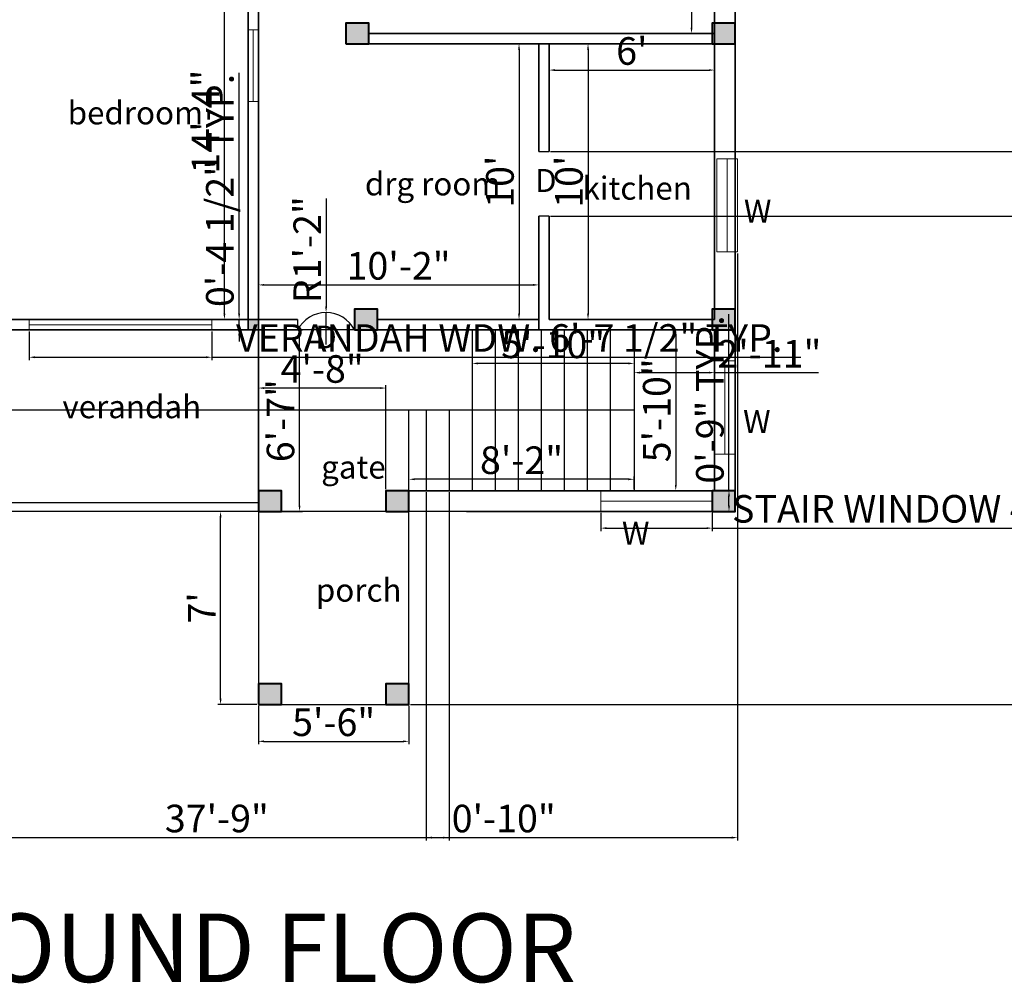
# Model space of a CAD drawing. Units: inches. Extents: x 1989 to 3287, y 1752 to 2384.
# Tile 2 of 5: x 2209 to 2638, y 1752 to 2172. Entities that reach past the tile are written whole.
import ezdxf

# ---------------------------------------------------------------- set-up
doc = ezdxf.new("R2010")
doc.units = ezdxf.units.IN
for name, color, linetype, lineweight in [('A-ANNO-DIMS', 2, 'Continuous', 18), ('A-ANNO-TEXT', 7, 'Continuous', 18), ('A-AREA-IDEN', 7, 'Continuous', 18), ('A-COLS', 1, 'Continuous', 40), ('A-COLS-PATT', 8, 'Continuous', 13), ('A-DOOR', 3, 'Continuous', 25), ('A-FLOR-EDGE', 7, 'Continuous', 25), ('A-FLOR-STRS', 7, 'Continuous', 25), ('A-GLAZ', 4, 'Continuous', 18), ('A-WALL', 7, 'Continuous', 35)]:
    doc.layers.add(name, color=color, linetype=linetype, lineweight=lineweight)
doc.styles.get("Standard").update_dxf_attribs({"font": 'arial.ttf'})
doc.dimstyles.new('ISO-25', dxfattribs={"dimtxt": 12, "dimasz": 2.5, "dimexe": 1.25, "dimexo": 0.625, "dimtad": 1, "dimdec": 0, "dimlunit": 4, "dimtxsty": 'Standard', "dimcen": 2.5, "dimadec": 0, "dimazin": 0, "dimtfac": 1, "dimtdec": 0, "dimtmove": 0, "dimatfit": 3, "dimfxl": 1, "dimarcsym": 0})

# ---------------------------------------------------------------- blocks, each defined once
blk = doc.blocks.new('*D1')
at = {"layer": 'A-ANNO-DIMS', "color": 0, "lineweight": -2, "transparency": 16777216}
for p, q in [((2312.51, 1957.68), (2295.45, 1957.68)), ((2296.7, 1876.18), (2296.7, 1955.18)), ((2312.51, 1873.68), (2295.45, 1873.68))]:
    blk.add_line(p, q, dxfattribs=at)
at = {"layer": 'A-ANNO-DIMS', "color": 0, "transparency": 16777216}
for points in [[(2296.28, 1955.18), (2297.11, 1955.18), (2296.7, 1957.68)], [(2296.28, 1876.18), (2297.11, 1876.18), (2296.7, 1873.68)]]:
    blk.add_solid(points, dxfattribs=at)
at = {"layer": 'Defpoints', "color": 0, "transparency": 16777216}
for p in [(2296.7, 1957.68), (2313.14, 1957.68), (2313.14, 1873.68)]:
    blk.add_point(p, dxfattribs=at)
at = {"layer": 'A-ANNO-DIMS', "color": 0, "transparency": 16777216, "insert": (2290.07, 1915.68), "char_height": 12, "attachment_point": 5, "rotation": 90}
blk.add_mtext("7'", dxfattribs=at)
blk = doc.blocks.new('*D2')
at = {"layer": 'A-ANNO-DIMS', "color": 0, "lineweight": -2, "transparency": 16777216}
for p, q in [((2313.14, 1873.05), (2313.14, 1856.37)), ((2378.64, 1873.05), (2378.64, 1856.37)), ((2315.64, 1857.62), (2376.14, 1857.62))]:
    blk.add_line(p, q, dxfattribs=at)
at = {"layer": 'A-ANNO-DIMS', "color": 0, "transparency": 16777216}
for points in [[(2315.64, 1858.04), (2315.64, 1857.2), (2313.14, 1857.62)], [(2376.14, 1858.04), (2376.14, 1857.2), (2378.64, 1857.62)]]:
    blk.add_solid(points, dxfattribs=at)
at = {"layer": 'Defpoints', "color": 0, "transparency": 16777216}
for p in [(2313.14, 1873.68), (2378.64, 1873.68), (2378.64, 1857.62)]:
    blk.add_point(p, dxfattribs=at)
at = {"layer": 'A-ANNO-DIMS', "color": 0, "transparency": 16777216, "insert": (2345.89, 1864.37), "char_height": 12, "attachment_point": 5}
blk.add_mtext('5\'-6"', dxfattribs=at)
blk = doc.blocks.new('*D3')
at = {"layer": 'A-ANNO-DIMS', "color": 0, "lineweight": -2, "transparency": 16777216}
for p, q in [((2476.64, 2029.77), (2476.64, 2016.83)), ((2511.64, 2029.77), (2511.64, 2016.83)), ((2479.14, 2018.08), (2509.14, 2018.08)), ((2511.64, 2018.08), (2556.81, 2018.08))]:
    blk.add_line(p, q, dxfattribs=at)
at = {"layer": 'A-ANNO-DIMS', "color": 0, "transparency": 16777216}
for points in [[(2479.14, 2018.5), (2479.14, 2017.67), (2476.64, 2018.08)], [(2509.14, 2018.5), (2509.14, 2017.67), (2511.64, 2018.08)]]:
    blk.add_solid(points, dxfattribs=at)
at = {"layer": 'Defpoints', "color": 0, "transparency": 16777216}
for p in [(2476.64, 2030.39), (2511.64, 2030.39), (2511.64, 2018.08)]:
    blk.add_point(p, dxfattribs=at)
at = {"layer": 'A-ANNO-DIMS', "color": 0, "transparency": 16777216, "insert": (2535.47, 2024.73), "char_height": 12, "attachment_point": 5}
blk.add_mtext('2\'-11"', dxfattribs=at)
blk = doc.blocks.new('*D4')
at = {"layer": 'A-ANNO-DIMS', "color": 0, "lineweight": -2, "transparency": 16777216}
for p, q in [((2477.26, 2036.68), (2496.01, 2036.68)), ((2494.76, 2034.18), (2494.76, 1969.18)), ((2477.26, 1966.68), (2496.01, 1966.68))]:
    blk.add_line(p, q, dxfattribs=at)
at = {"layer": 'A-ANNO-DIMS', "color": 0, "transparency": 16777216}
for points in [[(2494.34, 2034.18), (2495.17, 2034.18), (2494.76, 2036.68)], [(2494.34, 1969.18), (2495.17, 1969.18), (2494.76, 1966.68)]]:
    blk.add_solid(points, dxfattribs=at)
at = {"layer": 'Defpoints', "color": 0, "transparency": 16777216}
for p in [(2476.64, 2036.68), (2476.64, 1966.68), (2494.76, 1966.68)]:
    blk.add_point(p, dxfattribs=at)
at = {"layer": 'A-ANNO-DIMS', "color": 0, "transparency": 16777216, "insert": (2488.01, 2001.68), "char_height": 12, "attachment_point": 5, "rotation": 90}
blk.add_mtext('5\'-10"', dxfattribs=at)
blk = doc.blocks.new('*D5')
at = {"layer": 'A-ANNO-DIMS', "color": 0, "lineweight": -2, "transparency": 16777216}
for p, q in [((2406.14, 2036.05), (2406.14, 2020.84)), ((2476.64, 2036.05), (2476.64, 2020.84)), ((2474.14, 2022.09), (2408.64, 2022.09))]:
    blk.add_line(p, q, dxfattribs=at)
at = {"layer": 'A-ANNO-DIMS', "color": 0, "transparency": 16777216}
for points in [[(2408.64, 2022.5), (2408.64, 2021.67), (2406.14, 2022.09)], [(2474.14, 2022.5), (2474.14, 2021.67), (2476.64, 2022.09)]]:
    blk.add_solid(points, dxfattribs=at)
at = {"layer": 'Defpoints', "color": 0, "transparency": 16777216}
for p in [(2406.14, 2036.68), (2476.64, 2036.68), (2406.14, 2022.09)]:
    blk.add_point(p, dxfattribs=at)
at = {"layer": 'A-ANNO-DIMS', "color": 0, "transparency": 16777216, "insert": (2441.39, 2028.84), "char_height": 12, "attachment_point": 5}
blk.add_mtext('5\'-10"', dxfattribs=at)
blk = doc.blocks.new('*D6')
at = {"layer": 'A-ANNO-DIMS', "color": 0, "lineweight": -2, "transparency": 16777216}
for p, q in [((2378.64, 1967.3), (2378.64, 1972.92)), ((2474.14, 1971.67), (2381.14, 1971.67)), ((2476.64, 1967.3), (2476.64, 1972.92))]:
    blk.add_line(p, q, dxfattribs=at)
at = {"layer": 'A-ANNO-DIMS', "color": 0, "transparency": 16777216}
for points in [[(2381.14, 1972.08), (2381.14, 1971.25), (2378.64, 1971.67)], [(2474.14, 1972.08), (2474.14, 1971.25), (2476.64, 1971.67)]]:
    blk.add_solid(points, dxfattribs=at)
at = {"layer": 'Defpoints', "color": 0, "transparency": 16777216}
for p in [(2378.64, 1971.67), (2378.64, 1966.68), (2476.64, 1966.68)]:
    blk.add_point(p, dxfattribs=at)
at = {"layer": 'A-ANNO-DIMS', "color": 0, "transparency": 16777216, "insert": (2427.64, 1978.42), "char_height": 12, "attachment_point": 5}
blk.add_mtext('8\'-2"', dxfattribs=at)
blk = doc.blocks.new('*D7')
at = {"layer": 'A-ANNO-DIMS', "color": 0, "lineweight": -2, "transparency": 16777216}
for p, q in [((2313.14, 1967.3), (2313.14, 2012.61)), ((2366.14, 2011.36), (2315.64, 2011.36)), ((2368.64, 1967.3), (2368.64, 2012.61))]:
    blk.add_line(p, q, dxfattribs=at)
at = {"layer": 'A-ANNO-DIMS', "color": 0, "transparency": 16777216}
for points in [[(2315.64, 2011.78), (2315.64, 2010.95), (2313.14, 2011.36)], [(2366.14, 2011.78), (2366.14, 2010.95), (2368.64, 2011.36)]]:
    blk.add_solid(points, dxfattribs=at)
at = {"layer": 'Defpoints', "color": 0, "transparency": 16777216}
for p in [(2313.14, 2011.36), (2313.14, 1966.68), (2368.64, 1966.68)]:
    blk.add_point(p, dxfattribs=at)
at = {"layer": 'A-ANNO-DIMS', "color": 0, "transparency": 16777216, "insert": (2340.89, 2018.12), "char_height": 12, "attachment_point": 5}
blk.add_mtext('4\'-8"', dxfattribs=at)
blk = doc.blocks.new('*D8')
at = {"layer": 'A-ANNO-DIMS', "color": 0, "lineweight": -2, "transparency": 16777216}
for p, q in [((2313.76, 2036.68), (2332.3, 2036.68)), ((2331.05, 1960.18), (2331.05, 2034.18)), ((2313.76, 1957.68), (2332.3, 1957.68))]:
    blk.add_line(p, q, dxfattribs=at)
at = {"layer": 'A-ANNO-DIMS', "color": 0, "transparency": 16777216}
for points in [[(2330.64, 2034.18), (2331.47, 2034.18), (2331.05, 2036.68)], [(2330.64, 1960.18), (2331.47, 1960.18), (2331.05, 1957.68)]]:
    blk.add_solid(points, dxfattribs=at)
at = {"layer": 'Defpoints', "color": 0, "transparency": 16777216}
for p in [(2313.14, 2036.68), (2331.05, 2036.68), (2313.14, 1957.68)]:
    blk.add_point(p, dxfattribs=at)
at = {"layer": 'A-ANNO-DIMS', "color": 0, "transparency": 16777216, "insert": (2324.3, 1997.18), "char_height": 12, "attachment_point": 5, "rotation": 90}
blk.add_mtext('6\'-7"', dxfattribs=at)
blk = doc.blocks.new('*D9')
at = {"layer": 'A-ANNO-DIMS', "color": 0, "lineweight": -2, "transparency": 16777216}
for p, q in [((2308.01, 2213.45), (2297.11, 2213.45)), ((2298.36, 2043.68), (2298.36, 2210.95)), ((2308.01, 2041.18), (2297.11, 2041.18))]:
    blk.add_line(p, q, dxfattribs=at)
at = {"layer": 'A-ANNO-DIMS', "color": 0, "transparency": 16777216}
for points in [[(2297.94, 2210.95), (2298.78, 2210.95), (2298.36, 2213.45)], [(2297.94, 2043.68), (2298.78, 2043.68), (2298.36, 2041.18)]]:
    blk.add_solid(points, dxfattribs=at)
at = {"layer": 'Defpoints', "color": 0, "transparency": 16777216}
for p in [(2298.36, 2213.45), (2308.64, 2213.45), (2308.64, 2041.18)]:
    blk.add_point(p, dxfattribs=at)
at = {"layer": 'A-ANNO-DIMS', "color": 0, "transparency": 16777216, "insert": (2291.71, 2127.31), "char_height": 12, "attachment_point": 5, "rotation": 90}
blk.add_mtext('14\'-4"', dxfattribs=at)
blk = doc.blocks.new('*D13')
at = {"layer": 'A-ANNO-DIMS', "color": 0, "lineweight": -2, "transparency": 16777216}
for p, q in [((2511.01, 2297.68), (2500.35, 2297.68)), ((2501.6, 2295.18), (2501.6, 2168.18)), ((2511.01, 2165.68), (2500.35, 2165.68))]:
    blk.add_line(p, q, dxfattribs=at)
at = {"layer": 'A-ANNO-DIMS', "color": 0, "transparency": 16777216}
for points in [[(2501.18, 2295.18), (2502.02, 2295.18), (2501.6, 2297.68)], [(2501.18, 2168.18), (2502.02, 2168.18), (2501.6, 2165.68)]]:
    blk.add_solid(points, dxfattribs=at)
at = {"layer": 'Defpoints', "color": 0, "transparency": 16777216}
for p in [(2511.64, 2297.68), (2501.6, 2165.68), (2511.64, 2165.68)]:
    blk.add_point(p, dxfattribs=at)
at = {"layer": 'A-ANNO-DIMS', "color": 0, "transparency": 16777216, "insert": (2494.95, 2231.68), "char_height": 12, "attachment_point": 5, "rotation": 90}
blk.add_mtext("11'", dxfattribs=at)
blk = doc.blocks.new('*D35')
at = {"layer": 'A-ANNO-DIMS', "color": 0, "lineweight": -2, "transparency": 16777216}
for p, q in [((2439.64, 2160.55), (2439.64, 2148.49)), ((2511.64, 2160.55), (2511.64, 2148.49)), ((2442.14, 2149.74), (2509.14, 2149.74))]:
    blk.add_line(p, q, dxfattribs=at)
at = {"layer": 'A-ANNO-DIMS', "color": 0, "transparency": 16777216}
for points in [[(2442.14, 2150.16), (2442.14, 2149.32), (2439.64, 2149.74)], [(2509.14, 2150.16), (2509.14, 2149.32), (2511.64, 2149.74)]]:
    blk.add_solid(points, dxfattribs=at)
at = {"layer": 'Defpoints', "color": 0, "transparency": 16777216}
for p in [(2439.64, 2161.18), (2511.64, 2161.18), (2511.64, 2149.74)]:
    blk.add_point(p, dxfattribs=at)
at = {"layer": 'A-ANNO-DIMS', "color": 0, "transparency": 16777216, "insert": (2475.64, 2156.49), "char_height": 12, "attachment_point": 5}
blk.add_mtext("6'", dxfattribs=at)
blk = doc.blocks.new('*D36')
at = {"layer": 'A-ANNO-DIMS', "color": 0, "lineweight": -2, "transparency": 16777216}
for p, q in [((2440.26, 2161.18), (2457.82, 2161.18)), ((2456.57, 2158.68), (2456.57, 2043.68)), ((2440.26, 2041.18), (2457.82, 2041.18))]:
    blk.add_line(p, q, dxfattribs=at)
at = {"layer": 'A-ANNO-DIMS', "color": 0, "transparency": 16777216}
for points in [[(2456.16, 2158.68), (2456.99, 2158.68), (2456.57, 2161.18)], [(2456.16, 2043.68), (2456.99, 2043.68), (2456.57, 2041.18)]]:
    blk.add_solid(points, dxfattribs=at)
at = {"layer": 'Defpoints', "color": 0, "transparency": 16777216}
for p in [(2439.64, 2161.18), (2439.64, 2041.18), (2456.57, 2041.18)]:
    blk.add_point(p, dxfattribs=at)
at = {"layer": 'A-ANNO-DIMS', "color": 0, "transparency": 16777216, "insert": (2449.82, 2101.18), "char_height": 12, "attachment_point": 5, "rotation": 90}
blk.add_mtext("10'", dxfattribs=at)
blk = doc.blocks.new('*D37')
at = {"layer": 'A-ANNO-DIMS', "color": 0, "lineweight": -2, "transparency": 16777216}
for p, q in [((2313.14, 2041.8), (2313.14, 2057.5)), ((2435.14, 2041.8), (2435.14, 2057.5)), ((2315.64, 2056.25), (2432.64, 2056.25))]:
    blk.add_line(p, q, dxfattribs=at)
at = {"layer": 'A-ANNO-DIMS', "color": 0, "transparency": 16777216}
for points in [[(2315.64, 2056.66), (2315.64, 2055.83), (2313.14, 2056.25)], [(2432.64, 2056.66), (2432.64, 2055.83), (2435.14, 2056.25)]]:
    blk.add_solid(points, dxfattribs=at)
at = {"layer": 'Defpoints', "color": 0, "transparency": 16777216}
for p in [(2435.14, 2056.25), (2313.14, 2041.18), (2435.14, 2041.18)]:
    blk.add_point(p, dxfattribs=at)
at = {"layer": 'A-ANNO-DIMS', "color": 0, "transparency": 16777216, "insert": (2374.14, 2063), "char_height": 12, "attachment_point": 5}
blk.add_mtext('10\'-2"', dxfattribs=at)
blk = doc.blocks.new('*D38')
at = {"layer": 'A-ANNO-DIMS', "color": 0, "lineweight": -2, "transparency": 16777216}
for p, q in [((2434.51, 2161.18), (2425.3, 2161.18)), ((2426.55, 2158.68), (2426.55, 2043.68)), ((2434.51, 2041.18), (2425.3, 2041.18))]:
    blk.add_line(p, q, dxfattribs=at)
at = {"layer": 'A-ANNO-DIMS', "color": 0, "transparency": 16777216}
for points in [[(2426.13, 2158.68), (2426.97, 2158.68), (2426.55, 2161.18)], [(2426.13, 2043.68), (2426.97, 2043.68), (2426.55, 2041.18)]]:
    blk.add_solid(points, dxfattribs=at)
at = {"layer": 'Defpoints', "color": 0, "transparency": 16777216}
for p in [(2435.14, 2161.18), (2426.55, 2041.18), (2435.14, 2041.18)]:
    blk.add_point(p, dxfattribs=at)
at = {"layer": 'A-ANNO-DIMS', "color": 0, "transparency": 16777216, "insert": (2419.8, 2101.18), "char_height": 12, "attachment_point": 5, "rotation": 90}
blk.add_mtext("10'", dxfattribs=at)
blk = doc.blocks.new('WIN-EXT-STANDARD')
blk.add_line((4.5, 0), (4.5, 40.55))
blk.add_lwpolyline([(0, 40.55), (9, 40.55), (9, 0), (0, 0)], close=True)
blk = doc.blocks.new('WIN-STAIR-FRONT')
blk.add_line((0, 4.5), (48.49, 4.5))
blk.add_lwpolyline([(48.49, 9), (0, 9), (0, 0), (48.49, 0)], close=True)
blk = doc.blocks.new('WIN-BEDROOM-VERANDAH')
for p, q in [((0, 0), (0, 4.5)), ((79.39, 0), (79.39, 4.5)), ((0, 2.25), (79.39, 2.25))]:
    blk.add_line(p, q)
blk = doc.blocks.new('*D55')
at = {"layer": 'A-ANNO-DIMS', "color": 0, "lineweight": -2, "transparency": 16777216}
for p, q in [((2462.14, 1957.05), (2462.14, 1949.16)), ((2510.63, 1957.05), (2510.63, 1949.16)), ((2464.64, 1950.41), (2508.13, 1950.41)), ((2510.63, 1950.41), (2747.67, 1950.41))]:
    blk.add_line(p, q, dxfattribs=at)
at = {"layer": 'A-ANNO-DIMS', "color": 0, "transparency": 16777216}
for points in [[(2464.64, 1950.82), (2464.64, 1949.99), (2462.14, 1950.41)], [(2508.13, 1950.82), (2508.13, 1949.99), (2510.63, 1950.41)]]:
    blk.add_solid(points, dxfattribs=at)
at = {"layer": 'Defpoints', "color": 0, "transparency": 16777216}
for p in [(2462.14, 1957.68), (2510.63, 1957.68), (2510.63, 1950.41)]:
    blk.add_point(p, dxfattribs=at)
at = {"layer": 'A-ANNO-DIMS', "color": 0, "transparency": 16777216, "insert": (2630.4, 1957.24), "char_height": 12, "attachment_point": 5}
blk.add_mtext('STAIR WINDOW 4\'-0 1/2" TYP.', dxfattribs=at)
blk = doc.blocks.new('*D56')
at = {"layer": 'A-ANNO-DIMS', "color": 0, "lineweight": -2, "transparency": 16777216}
for p, q in [((2517.9, 1966.68), (2517.9, 2043.58)), ((2511.26, 1966.68), (2519.15, 1966.68)), ((2517.9, 1960.18), (2517.9, 1964.18)), ((2511.26, 1957.68), (2519.15, 1957.68))]:
    blk.add_line(p, q, dxfattribs=at)
at = {"layer": 'A-ANNO-DIMS', "color": 0, "transparency": 16777216}
for points in [[(2517.49, 1964.18), (2518.32, 1964.18), (2517.9, 1966.68)], [(2517.49, 1960.18), (2518.32, 1960.18), (2517.9, 1957.68)]]:
    blk.add_solid(points, dxfattribs=at)
at = {"layer": 'Defpoints', "color": 0, "transparency": 16777216}
for p in [(2510.63, 1966.68), (2517.9, 1966.68), (2510.63, 1957.68)]:
    blk.add_point(p, dxfattribs=at)
at = {"layer": 'A-ANNO-DIMS', "color": 0, "transparency": 16777216, "insert": (2511.15, 2006.38), "char_height": 12, "attachment_point": 5, "rotation": 90}
blk.add_mtext('0\'-9" TYP.', dxfattribs=at)
blk = doc.blocks.new('*D59')
at = {"layer": 'A-ANNO-DIMS', "color": 0, "lineweight": -2, "transparency": 16777216}
for p, q in [((2213.46, 2036.05), (2213.46, 2023.52)), ((2292.85, 2036.05), (2292.85, 2023.52)), ((2215.96, 2024.77), (2290.35, 2024.77)), ((2292.85, 2024.77), (2549.21, 2024.77))]:
    blk.add_line(p, q, dxfattribs=at)
at = {"layer": 'A-ANNO-DIMS', "color": 0, "transparency": 16777216}
for points in [[(2215.96, 2025.19), (2215.96, 2024.35), (2213.46, 2024.77)], [(2290.35, 2025.19), (2290.35, 2024.35), (2292.85, 2024.77)]]:
    blk.add_solid(points, dxfattribs=at)
at = {"layer": 'Defpoints', "color": 0, "transparency": 16777216}
for p in [(2213.46, 2036.68), (2292.85, 2036.68), (2292.85, 2024.77)]:
    blk.add_point(p, dxfattribs=at)
at = {"layer": 'A-ANNO-DIMS', "color": 0, "transparency": 16777216, "insert": (2422.28, 2031.6), "char_height": 12, "attachment_point": 5}
blk.add_mtext('VERANDAH WDW. 6\'-7 1/2" TYP.', dxfattribs=at)
blk = doc.blocks.new('*D60')
at = {"layer": 'A-ANNO-DIMS', "color": 0, "lineweight": -2, "transparency": 16777216}
for p, q in [((2304.76, 2043.68), (2304.76, 2148.54)), ((2293.48, 2041.18), (2306.01, 2041.18)), ((2304.76, 2036.68), (2304.76, 2041.18)), ((2293.48, 2036.68), (2306.01, 2036.68)), ((2304.76, 2034.18), (2304.76, 2031.68))]:
    blk.add_line(p, q, dxfattribs=at)
at = {"layer": 'A-ANNO-DIMS', "color": 0, "transparency": 16777216}
for points in [[(2304.34, 2043.68), (2305.18, 2043.68), (2304.76, 2041.18)], [(2304.34, 2034.18), (2305.18, 2034.18), (2304.76, 2036.68)]]:
    blk.add_solid(points, dxfattribs=at)
at = {"layer": 'Defpoints', "color": 0, "transparency": 16777216}
for p in [(2292.85, 2041.18), (2304.76, 2041.18), (2292.85, 2036.68)]:
    blk.add_point(p, dxfattribs=at)
at = {"layer": 'A-ANNO-DIMS', "color": 0, "transparency": 16777216, "insert": (2297.93, 2097.36), "char_height": 12, "attachment_point": 5, "rotation": 90}
blk.add_mtext('0\'-4 1/2" TYP.', dxfattribs=at)
blk = doc.blocks.new('*D63')
at = {"layer": 'A-ANNO-DIMS', "color": 0, "lineweight": -2, "transparency": 16777216}
for p, q in [((2521.64, 2069.99), (2521.64, 1814.48)), ((2068.49, 1892.56), (2068.49, 1814.48)), ((2070.99, 1815.73), (2519.14, 1815.73))]:
    blk.add_line(p, q, dxfattribs=at)
at = {"layer": 'A-ANNO-DIMS', "color": 0, "transparency": 16777216}
for points in [[(2070.99, 1816.15), (2070.99, 1815.31), (2068.49, 1815.73)], [(2519.14, 1816.15), (2519.14, 1815.31), (2521.64, 1815.73)]]:
    blk.add_solid(points, dxfattribs=at)
at = {"layer": 'Defpoints', "color": 0, "transparency": 16777216}
for p in [(2521.64, 2070.62), (2068.49, 1893.19), (2521.64, 1815.73)]:
    blk.add_point(p, dxfattribs=at)
at = {"layer": 'A-ANNO-DIMS', "color": 0, "transparency": 16777216, "insert": (2295.06, 1822.49), "char_height": 12, "attachment_point": 5}
blk.add_mtext('37\'-9"', dxfattribs=at)
blk = doc.blocks.new('*D64')
at = {"layer": 'A-ANNO-DIMS', "color": 0, "lineweight": -2, "transparency": 16777216}
for p, q in [((2521.26, 2306.68), (3180.41, 2306.68)), ((3179.16, 1876.18), (3179.16, 2304.18)), ((2379.26, 1873.68), (3180.41, 1873.68))]:
    blk.add_line(p, q, dxfattribs=at)
at = {"layer": 'A-ANNO-DIMS', "color": 0, "transparency": 16777216}
for points in [[(3178.74, 2304.18), (3179.58, 2304.18), (3179.16, 2306.68)], [(3178.74, 1876.18), (3179.58, 1876.18), (3179.16, 1873.68)]]:
    blk.add_solid(points, dxfattribs=at)
at = {"layer": 'Defpoints', "color": 0, "transparency": 16777216}
for p in [(2520.64, 2306.68), (3179.16, 2306.68), (2378.64, 1873.68)]:
    blk.add_point(p, dxfattribs=at)
at = {"layer": 'A-ANNO-DIMS', "color": 0, "transparency": 16777216, "insert": (3172.4, 2090.18), "char_height": 12, "attachment_point": 5, "rotation": 90}
blk.add_mtext('36\'-1"', dxfattribs=at)
blk = doc.blocks.new('*D74')
at = {"layer": 'A-ANNO-DIMS', "color": 0, "lineweight": -2, "transparency": 16777216}
for p, q in [((3179.16, 2114.35), (3179.16, 2150.2)), ((2440.26, 2114.35), (3180.41, 2114.35)), ((3179.16, 2088.6), (3179.16, 2111.85)), ((2440.26, 2086.1), (3180.41, 2086.1))]:
    blk.add_line(p, q, dxfattribs=at)
at = {"layer": 'A-ANNO-DIMS', "color": 0, "transparency": 16777216}
for points in [[(3178.74, 2111.85), (3179.58, 2111.85), (3179.16, 2114.35)], [(3178.74, 2088.6), (3179.58, 2088.6), (3179.16, 2086.1)]]:
    blk.add_solid(points, dxfattribs=at)
at = {"layer": 'Defpoints', "color": 0, "transparency": 16777216}
for p in [(2439.64, 2114.35), (3179.16, 2114.35), (2439.64, 2086.1)]:
    blk.add_point(p, dxfattribs=at)
at = {"layer": 'A-ANNO-DIMS', "color": 0, "transparency": 16777216, "insert": (3172.51, 2133.53), "char_height": 12, "attachment_point": 5, "rotation": 90}
blk.add_mtext('2\'-4"', dxfattribs=at)
blk = doc.blocks.new('*D76')
at = {"layer": 'A-ANNO-DIMS', "color": 0, "lineweight": -2, "transparency": 16777216}
for p, q in [((2386.14, 1966.05), (2386.14, 1814.48)), ((2396.14, 1966.05), (2396.14, 1814.48)), ((2388.64, 1815.73), (2393.64, 1815.73)), ((2396.14, 1815.73), (2441.11, 1815.73))]:
    blk.add_line(p, q, dxfattribs=at)
at = {"layer": 'A-ANNO-DIMS', "color": 0, "transparency": 16777216}
for points in [[(2388.64, 1816.15), (2388.64, 1815.31), (2386.14, 1815.73)], [(2393.64, 1816.15), (2393.64, 1815.31), (2396.14, 1815.73)]]:
    blk.add_solid(points, dxfattribs=at)
at = {"layer": 'Defpoints', "color": 0, "transparency": 16777216}
for p in [(2386.14, 1966.68), (2396.14, 1966.68), (2396.14, 1815.73)]:
    blk.add_point(p, dxfattribs=at)
at = {"layer": 'A-ANNO-DIMS', "color": 0, "transparency": 16777216, "insert": (2419.88, 1822.48), "char_height": 12, "attachment_point": 5}
blk.add_mtext('0\'-10"', dxfattribs=at)
blk = doc.blocks.new('*D77')
at = {"layer": 'A-ANNO-DIMS', "color": 0, "lineweight": -2, "transparency": 16777216}
for p, q in [((2013.54, 2036.68), (2013.54, 2081.86)), ((2405.51, 2036.68), (2012.29, 2036.68)), ((2013.54, 2004.18), (2013.54, 2034.18)), ((2395.51, 2001.68), (2012.29, 2001.68))]:
    blk.add_line(p, q, dxfattribs=at)
at = {"layer": 'A-ANNO-DIMS', "color": 0, "transparency": 16777216}
for points in [[(2013.12, 2034.18), (2013.95, 2034.18), (2013.54, 2036.68)], [(2013.12, 2004.18), (2013.95, 2004.18), (2013.54, 2001.68)]]:
    blk.add_solid(points, dxfattribs=at)
at = {"layer": 'Defpoints', "color": 0, "transparency": 16777216}
for p in [(2013.54, 2036.68), (2406.14, 2036.68), (2396.14, 2001.68)]:
    blk.add_point(p, dxfattribs=at)
at = {"layer": 'A-ANNO-DIMS', "color": 0, "transparency": 16777216, "insert": (2006.89, 2060.52), "char_height": 12, "attachment_point": 5, "rotation": 90}
blk.add_mtext('2\'-11"', dxfattribs=at)
blk = doc.blocks.new('*D78')
at = {"layer": 'A-ANNO-DIMS', "color": 0, "lineweight": -2, "transparency": 16777216}
for p, q in [((2342.6, 2093.89), (2342.6, 2046.75)), ((2342.6, 2030.33), (2342.6, 2044.25))]:
    blk.add_line(p, q, dxfattribs=at)
at = {"layer": 'A-ANNO-DIMS', "color": 0, "transparency": 16777216}
blk.add_solid([(2342.18, 2046.75), (2343.02, 2046.75), (2342.6, 2044.25)], dxfattribs=at)
at = {"layer": 'Defpoints', "color": 0, "transparency": 16777216}
for p in [(2342.6, 2044.25), (2342.6, 2030.33)]:
    blk.add_point(p, dxfattribs=at)
at = {"layer": 'A-ANNO-DIMS', "color": 0, "transparency": 16777216, "insert": (2335.95, 2071.57), "char_height": 12, "attachment_point": 5, "rotation": 89.9989}
blk.add_mtext('R1\'-2"', dxfattribs=at)

msp = doc.modelspace()

# ---------------------------------------------------------------- hatches: boundary and pattern name
at = {"layer": 'A-COLS-PATT'}
h = msp.add_hatch(dxfattribs=at)
h.set_pattern_fill('GRAVEL', color=256, scale=0.2)
h.paths.add_polyline_path([(3123.21, 2045.68), (3114.21, 2045.68), (3114.21, 2041.18), (3113.21, 2041.18), (3113.21, 2036.68), (3123.21, 2036.68)])
h.paths.add_polyline_path([(2962.75, 2170.18), (2952.75, 2170.18), (2952.75, 2161.18), (2962.75, 2161.18)])
h.paths.add_polyline_path([(2520.59, 2306.68), (2510.59, 2306.68), (2510.59, 2297.68), (2520.59, 2297.68)])
h.paths.add_polyline_path([(2520.64, 2170.18), (2511.64, 2170.18), (2511.64, 2161.18), (2520.64, 2161.18)])
h.paths.add_polyline_path([(2364.99, 2045.68), (2354.99, 2045.68), (2354.99, 2036.68), (2364.99, 2036.68)])
h.paths.add_polyline_path([(2361.14, 2170.18), (2351.14, 2170.18), (2351.14, 2161.18), (2361.14, 2161.18)])
h = msp.add_hatch(dxfattribs=at)
h.set_pattern_fill('GRAVEL', color=256, scale=0.2)
h.paths.add_polyline_path([(2520.64, 2045.68), (2511.64, 2045.68), (2511.64, 2041.18), (2510.64, 2041.18), (2510.64, 2036.68), (2520.64, 2036.68)])
h.paths.add_polyline_path([(2520.63, 1966.68), (2510.63, 1966.68), (2510.63, 1957.68), (2520.63, 1957.68)])
h.paths.add_polyline_path([(2323.14, 1882.68), (2313.14, 1882.68), (2313.14, 1873.68), (2323.14, 1873.68)])
h.paths.add_polyline_path([(2378.64, 1882.68), (2368.64, 1882.68), (2368.64, 1873.68), (2378.64, 1873.68)])
h.paths.add_polyline_path([(2378.64, 1966.68), (2368.64, 1966.68), (2368.64, 1957.68), (2378.64, 1957.68)])
h.paths.add_polyline_path([(2323.14, 1966.68), (2313.14, 1966.68), (2313.14, 1957.68), (2323.14, 1957.68)])
h.paths.add_polyline_path([(2313.14, 2041.18), (2308.64, 2041.18), (2308.64, 2036.68), (2313.14, 2036.68)])
h.paths.add_polyline_path([(2304.29, 2102.44), (2304.29, 2151.15), (2279.56, 2151.15), (2279.56, 2102.44)], flags=9)
h.paths.add_polyline_path([(2216.76, 2191.62), (2265.47, 2191.62), (2265.47, 2216.35), (2216.76, 2216.35)], flags=9)
h.paths.add_polyline_path([(2507.53, 2217.24), (2507.53, 2245.08), (2482.8, 2245.08), (2482.8, 2217.24)], flags=9)
h.paths.add_polyline_path([(2466.45, 2144.02), (2484.98, 2144.02), (2484.98, 2168.75), (2466.45, 2168.75)], flags=9)
h.paths.add_polyline_path([(2462.3, 2086.74), (2462.3, 2114.58), (2437.57, 2114.58), (2437.57, 2086.74)], flags=9)
h.paths.add_polyline_path([(2349.26, 2050.52), (2397.97, 2050.52), (2397.97, 2075.25), (2349.26, 2075.25)], flags=9)
h.paths.add_polyline_path([(2432.27, 2086.74), (2432.27, 2114.58), (2407.54, 2114.58), (2407.54, 2086.74)], flags=9)
h.paths.add_polyline_path([(2304.67, 2184.6), (2319.75, 2184.6), (2319.75, 2205.2), (2304.67, 2205.2)], flags=9)
h.paths.add_polyline_path([(2345.88, 2187.62), (2360.97, 2187.62), (2360.97, 2208.22), (2345.88, 2208.22)], flags=9)
h.paths.add_polyline_path([(2429.95, 2091.23), (2445.03, 2091.23), (2445.03, 2111.84), (2429.95, 2111.84)], flags=9)
h.paths.add_polyline_path([(2346.78, 2233.62), (2361.86, 2233.62), (2361.86, 2254.22), (2346.78, 2254.22)], flags=9)
h.paths.add_polyline_path([(2222.31, 2236.18), (2237.39, 2236.18), (2237.39, 2256.78), (2222.31, 2256.78)], flags=9)
h.paths.add_polyline_path([(2186.25, 2233.03), (2201.34, 2233.03), (2201.34, 2253.64), (2186.25, 2253.64)], flags=9)
h.paths.add_polyline_path([(2356.5, 2089.75), (2417.39, 2089.75), (2417.39, 2110.36), (2356.5, 2110.36)], flags=9)
h.paths.add_polyline_path([(2450.78, 2087.89), (2500.04, 2087.89), (2500.04, 2108.49), (2450.78, 2108.49)], flags=9)
h.paths.add_polyline_path([(2226.77, 2120.65), (2286.89, 2120.65), (2286.89, 2141.25), (2226.77, 2141.25)], flags=9)
h.paths.add_polyline_path([(2422.03, 2219.06), (2486.03, 2219.06), (2486.03, 2239.67), (2422.03, 2239.67)], flags=9)
h.paths.add_polyline_path([(2321.5, 2262.24), (2341.25, 2262.24), (2341.25, 2282.84), (2321.5, 2282.84)], flags=9)
h.paths.add_polyline_path([(2234.58, 2262.24), (2266.77, 2262.24), (2266.77, 2282.84), (2234.58, 2282.84)], flags=9)
h.paths.add_polyline_path([(2179.85, 2262.24), (2199.6, 2262.24), (2199.6, 2282.84), (2179.85, 2282.84)], flags=9)

# ---------------------------------------------------------------- linework, layer by layer
at = {"layer": 'A-COLS'}
for p, q in [((2351.14, 2170.18), (2351.14, 2161.18)), ((2364.99, 2045.68), (2354.99, 2045.68)), ((2354.99, 2045.68), (2354.99, 2036.68)), ((2323.14, 1966.68), (2313.14, 1966.68)), ((2378.64, 1966.68), (2368.64, 1966.68)), ((2368.64, 1966.68), (2368.64, 1957.68)), ((2378.64, 1882.68), (2368.64, 1882.68)), ((2368.64, 1882.68), (2368.64, 1873.68))]:
    msp.add_line(p, q, dxfattribs=at)
for points in [[(2351.14, 2161.18), (2361.14, 2161.18), (2361.14, 2170.18), (2351.14, 2170.18)], [(2510.65, 2161.18), (2520.65, 2161.18), (2520.65, 2170.18), (2510.65, 2170.18)], [(2354.99, 2036.68), (2364.99, 2036.68), (2364.99, 2045.68), (2354.99, 2045.68)], [(2510.64, 2036.68), (2520.64, 2036.68), (2520.64, 2045.68), (2510.64, 2045.68)], [(2313.14, 1957.68), (2323.14, 1957.68), (2323.14, 1966.68), (2313.14, 1966.68)], [(2368.64, 1957.68), (2378.64, 1957.68), (2378.64, 1966.68), (2368.64, 1966.68)], [(2510.63, 1957.68), (2520.63, 1957.68), (2520.63, 1966.68), (2510.63, 1966.68)], [(2313.14, 1873.68), (2323.14, 1873.68), (2323.14, 1882.68), (2313.14, 1882.68)], [(2368.64, 1873.68), (2378.64, 1873.68), (2378.64, 1882.68), (2368.64, 1882.68)]]:
    msp.add_lwpolyline(points, close=True, dxfattribs=at)
at = {"layer": 'A-DOOR'}
msp.add_line((2330.21, 2041.18), (2330.21, 2036.68), dxfattribs=at)
for points in [[(2435.14, 2114.35), (2439.64, 2114.35)], [(2439.64, 2086.1), (2435.14, 2086.1)]]:
    msp.add_lwpolyline(points, dxfattribs=at)
msp.add_arc((2342.6, 2030.33), 13.92, 27.1255, 152.8745, dxfattribs=at)
at = {"layer": 'A-FLOR-EDGE'}
for p, q in [((2378.64, 1873.68), (2378.64, 1962.18)), ((2174.64, 1961.55), (2313.14, 1961.55)), ((2312.64, 1957.68), (2174.64, 1957.68)), ((2413.64, 1957.68), (2312.64, 1957.68)), ((2313.14, 1957.68), (2313.14, 1873.68)), ((2313.14, 1873.68), (2378.64, 1873.68))]:
    msp.add_line(p, q, dxfattribs=at)
at = {"layer": 'A-FLOR-STRS'}
for p, q in [((2476.64, 2036.68), (2397.64, 2036.68)), ((2406.14, 2036.68), (2406.14, 1966.68)), ((2416.14, 2036.68), (2416.14, 1966.68)), ((2426.14, 2036.68), (2426.14, 1966.68)), ((2436.14, 2036.68), (2436.14, 1966.68)), ((2446.14, 2036.68), (2446.14, 1966.68)), ((2456.14, 2036.68), (2456.14, 1966.68)), ((2466.14, 2036.68), (2466.14, 1966.68)), ((2476.64, 2036.68), (2476.64, 1966.68)), ((2476.64, 2001.68), (2378.64, 2001.68)), ((2378.64, 1966.68), (2378.64, 2001.68)), ((2386.14, 2001.68), (2386.14, 1966.68)), ((2396.14, 2001.68), (2396.14, 1966.68)), ((2476.64, 1966.68), (2378.64, 1966.68))]:
    msp.add_line(p, q, dxfattribs=at)
at = {"layer": 'A-GLAZ'}
msp.add_line((2310.89, 2136.11), (2310.89, 2167.31), dxfattribs=at)
msp.add_lwpolyline([(2308.64, 2167.31), (2313.14, 2167.31), (2313.14, 2136.11), (2308.64, 2136.11)], close=True, dxfattribs=at)
at = {"layer": 'A-WALL'}
for p, q in [((2308.64, 2177.45), (2308.64, 2099.68)), ((2313.14, 2177.45), (2313.14, 2099.68)), ((2361.14, 2165.68), (2511.64, 2165.68)), ((2351.14, 2161.18), (2511.64, 2161.18)), ((2435.14, 2114.35), (2435.14, 2161.18)), ((2439.64, 2114.35), (2439.64, 2161.18)), ((2511.64, 2161.18), (2511.64, 2041.18)), ((2520.64, 2161.18), (2520.64, 2036.68)), ((2313.14, 2099.68), (2313.14, 1966.68)), ((2308.64, 2090.68), (2308.64, 2041.18)), ((2435.14, 2036.68), (2435.14, 2086.1)), ((2439.64, 2041.18), (2439.64, 2086.1)), ((2299.29, 2041.18), (2174.64, 2041.18)), ((2330.21, 2041.18), (2299.29, 2041.18)), ((2308.64, 2041.18), (2308.64, 2036.68)), ((2435.14, 2041.18), (2364.99, 2041.18)), ((2511.64, 2041.18), (2439.64, 2041.18)), ((2302.64, 2036.68), (2174.64, 2036.68)), ((2330.21, 2036.68), (2302.64, 2036.68)), ((2403.64, 2036.68), (2354.99, 2036.68)), ((2413.64, 2036.68), (2403.64, 2036.68)), ((2403.64, 2036.68), (2403.64, 2036.68)), ((2413.64, 2036.68), (2464.48, 2036.68)), ((2511.64, 2036.68), (2435.14, 2036.68)), ((2511.64, 2036.68), (2476.64, 2036.68)), ((2511.64, 2036.68), (2511.64, 1966.68)), ((2520.64, 2036.68), (2520.64, 1957.68)), ((2403.64, 1966.68), (2368.64, 1966.68)), ((2511.64, 1966.68), (2413.64, 1966.68)), ((2520.64, 1957.68), (2403.64, 1957.68))]:
    msp.add_line(p, q, dxfattribs=at)
for points in [[(2520.64, 2090.68), (2520.64, 2306.68), (2134.64, 2306.68), (2134.64, 2137.49)], [(2511.64, 2099.68), (2511.64, 2297.68), (2143.64, 2297.68)], [(2308.64, 2090.68), (2308.64, 2099.68)], [(2313.14, 2099.68), (2313.14, 2090.68)], [(2413.64, 1966.68), (2403.64, 1966.68)], [(2403.64, 1957.68), (2413.64, 1957.68)]]:
    msp.add_lwpolyline(points, dxfattribs=at)

# ---------------------------------------------------------------- block references
at = {"layer": 'A-GLAZ'}
for name, p in [('WIN-EXT-STANDARD', (2512.64, 2070.62)), ('WIN-BEDROOM-VERANDAH', (2213.46, 2036.68)), ('WIN-EXT-STANDARD', (2511.64, 1982.63)), ('WIN-STAIR-FRONT', (2462.14, 1957.68))]:
    msp.add_blockref(name, p, dxfattribs=at)

# ---------------------------------------------------------------- texts
at = {"layer": 'A-ANNO-TEXT', "attachment_point": 1}
for s, width, gutter_width, heights, insert, char_height in [('D', 78.3523, 49.99, [0], (2433.52, 2106.69), 10), ('W', 78.3523, 49.99, [0], (2524.4, 2093.35), 10), ('D', 78.3523, 49.99, [0], (2337.85, 2038.54), 10), ('W', 78.3523, 49.99, [0], (2524.04, 2001.75), 10), ('gate', 78.3523, 49.99, [10.16], (2340.46, 1981.97), 9.998), ('W', 78.3523, 49.99, [0], (2471.33, 1953.17), 10), ('GROUND FLOOR', 4273.6475, 149.09, [0], (2140.81, 1782.67), 29.8187)]:
    msp.add_mtext_dynamic_manual_height_columns(s, width=width, gutter_width=gutter_width, heights=heights, dxfattribs=dict(at, insert=insert, char_height=char_height))
at = {"layer": 'A-AREA-IDEN', "char_height": 9.998, "attachment_point": 1}
for s, insert in [('bedroom', (2230.18, 2136.11)), ('drg room', (2359.48, 2105.21)), ('kitchen', (2454.21, 2103.35)), ('verandah', (2227.87, 2008.24)), ('porch', (2338.15, 1928.41))]:
    msp.add_mtext_dynamic_manual_height_columns(s, width=78.3523, gutter_width=49.99, heights=[0], dxfattribs=dict(at, insert=insert))

# ---------------------------------------------------------------- dimensions: what is measured, and where the dimension line sits
at = {"layer": 'A-ANNO-DIMS'}
for base, p1, p2, override, picture, middle in [((3179.16, 2306.68), (2378.64, 1873.68), (2520.64, 2306.68), {"dimdec": 1, "dimlfac": 1, "dimrnd": 0, "dimzin": 1, "dimdsep": 46, "dimlunit": 4, "dimfrac": 2}, '*D64', (3172.4, 2090.18)), ((2501.6, 2165.68), (2511.64, 2297.68), (2511.64, 2165.68), {"dimclrd": 0, "dimclre": 0, "dimclrt": 0}, '*D13', (2494.95, 2231.68)), ((2298.36, 2213.45), (2308.64, 2041.18), (2308.64, 2213.45), {"dimclrd": 0, "dimclre": 0, "dimclrt": 0}, '*D9', (2291.71, 2127.31)), ((2426.55, 2041.18), (2435.14, 2161.18), (2435.14, 2041.18), {"dimclrd": 0, "dimclre": 0, "dimclrt": 0}, '*D38', (2419.8, 2101.18)), ((2456.57, 2041.18), (2439.64, 2161.18), (2439.64, 2041.18), {"dimclrd": 0, "dimclre": 0, "dimclrt": 0}, '*D36', (2449.82, 2101.18)), ((3179.1591, 2114.3493), (2439.6365, 2086.1013), (2439.6365, 2114.3493), {"dimdec": 1, "dimlfac": 1, "dimrnd": 0, "dimzin": 1, "dimdsep": 46, "dimlunit": 4, "dimfrac": 2}, '*D74', (3172.5095, 2133.5261)), ((2013.54, 2036.68), (2396.14, 2001.68), (2406.14, 2036.68), {"dimdec": 1, "dimlfac": 1, "dimrnd": 0, "dimzin": 1, "dimdsep": 46, "dimlunit": 4, "dimfrac": 2}, '*D77', (2006.89, 2060.52)), ((2331.05, 2036.68), (2313.14, 1957.68), (2313.14, 2036.68), {"dimclrd": 0, "dimclre": 0, "dimclrt": 0}, '*D8', (2324.3, 1997.18)), ((2494.76, 1966.68), (2476.64, 2036.68), (2476.64, 1966.68), {"dimclrd": 0, "dimclre": 0, "dimclrt": 0}, '*D4', (2488.01, 2001.68)), ((2296.7, 1957.68), (2313.14, 1873.68), (2313.14, 1957.68), {"dimclrd": 0, "dimclre": 0, "dimclrt": 0}, '*D1', (2290.07, 1915.68))]:
    dim = msp.add_linear_dim(base=base, p1=p1, p2=p2, angle=90, dimstyle='ISO-25', override=override, dxfattribs=at)
    dim.commit()
    dim.dimension.update_dxf_attribs({"geometry": picture, "text_midpoint": middle})
for base, p1, p2, override, picture, middle in [((2511.64, 2149.74), (2439.64, 2161.18), (2511.64, 2161.18), {"dimclrd": 0, "dimclre": 0, "dimclrt": 0}, '*D35', (2475.64, 2156.49)), ((2521.6365, 1815.73), (2068.4852, 1893.1857), (2521.6365, 2070.6179), {"dimdec": 1, "dimlfac": 1, "dimrnd": 0, "dimzin": 1, "dimdsep": 46, "dimlunit": 4, "dimfrac": 2}, '*D63', (2295.0609, 1822.486)), ((2435.14, 2056.25), (2313.14, 2041.18), (2435.14, 2041.18), {"dimclrd": 0, "dimclre": 0, "dimclrt": 0}, '*D37', (2374.14, 2063)), ((2406.1392, 2022.0856), (2476.6365, 2036.68), (2406.1392, 2036.68), {"dimclrd": 0, "dimclre": 0, "dimclrt": 0}, '*D5', (2441.3878, 2028.8375)), ((2511.64, 2018.08), (2476.64, 2030.39), (2511.64, 2030.39), {"dimclrd": 0, "dimclre": 0, "dimclrt": 0}, '*D3', (2535.47, 2024.73)), ((2313.13646977, 2011.36319293), (2368.63646977, 1966.67998165), (2313.13646977, 1966.67998165), {"dimclrd": 0, "dimclre": 0, "dimclrt": 0}, '*D7', (2340.88646977, 2018.11506878)), ((2378.64, 1971.67), (2476.64, 1966.68), (2378.64, 1966.68), {"dimclrd": 0, "dimclre": 0, "dimclrt": 0}, '*D6', (2427.64, 1978.42)), ((2396.14, 1815.73), (2386.14, 1966.68), (2396.14, 1966.68), {"dimdec": 1, "dimlfac": 1, "dimrnd": 0, "dimzin": 1, "dimdsep": 46, "dimlunit": 4, "dimfrac": 2}, '*D76', (2419.88, 1822.48)), ((2378.63646977, 1857.62054686), (2313.13646977, 1873.67998165), (2378.63646977, 1873.67998165), {"dimclrd": 0, "dimclre": 0, "dimclrt": 0}, '*D2', (2345.88646977, 1864.37242271))]:
    dim = msp.add_linear_dim(base=base, p1=p1, p2=p2, dimstyle='ISO-25', override=override, dxfattribs=at)
    dim.commit()
    dim.dimension.update_dxf_attribs({"geometry": picture, "text_midpoint": middle})
for base, p1, p2, picture, middle in [((2304.76, 2041.18), (2292.85, 2036.68), (2292.85, 2041.18), '*D60', (2297.93, 2097.36)), ((2517.9, 1966.68), (2510.63, 1957.68), (2510.63, 1966.68), '*D56', (2511.15, 2006.38))]:
    dim = msp.add_linear_dim(base=base, p1=p1, p2=p2, angle=90, text='<> TYP.', dimstyle='ISO-25', override={"dimdec": 1, "dimlfac": 1, "dimrnd": 0, "dimzin": 1, "dimdsep": 46, "dimlunit": 4, "dimfrac": 2}, dxfattribs=at)
    dim.commit()
    dim.dimension.update_dxf_attribs({"geometry": picture, "text_midpoint": middle})
dim = msp.add_radius_dim(center=(2342.6, 2030.33), mpoint=(2342.6, 2044.25), dimstyle='ISO-25', override={"dimdec": 1, "dimlfac": 1, "dimrnd": 0, "dimzin": 1, "dimdsep": 46, "dimlunit": 4, "dimfrac": 2}, dxfattribs=at)
dim.commit()
dim.dimension.update_dxf_attribs({"geometry": '*D78', "text_midpoint": (2335.95, 2071.57)})
for base, p1, p2, text, picture, middle in [((2292.85, 2024.77), (2213.46, 2036.68), (2292.85, 2036.68), 'VERANDAH WDW. <> TYP.', '*D59', (2422.28, 2031.6)), ((2510.63, 1950.41), (2462.14, 1957.68), (2510.63, 1957.68), 'STAIR WINDOW <> TYP.', '*D55', (2630.4, 1957.24))]:
    dim = msp.add_linear_dim(base=base, p1=p1, p2=p2, text=text, dimstyle='ISO-25', override={"dimdec": 1, "dimlfac": 1, "dimrnd": 0, "dimzin": 1, "dimdsep": 46, "dimlunit": 4, "dimfrac": 2}, dxfattribs=at)
    dim.commit()
    dim.dimension.update_dxf_attribs({"geometry": picture, "text_midpoint": middle})

doc.saveas('drawing.dxf')
